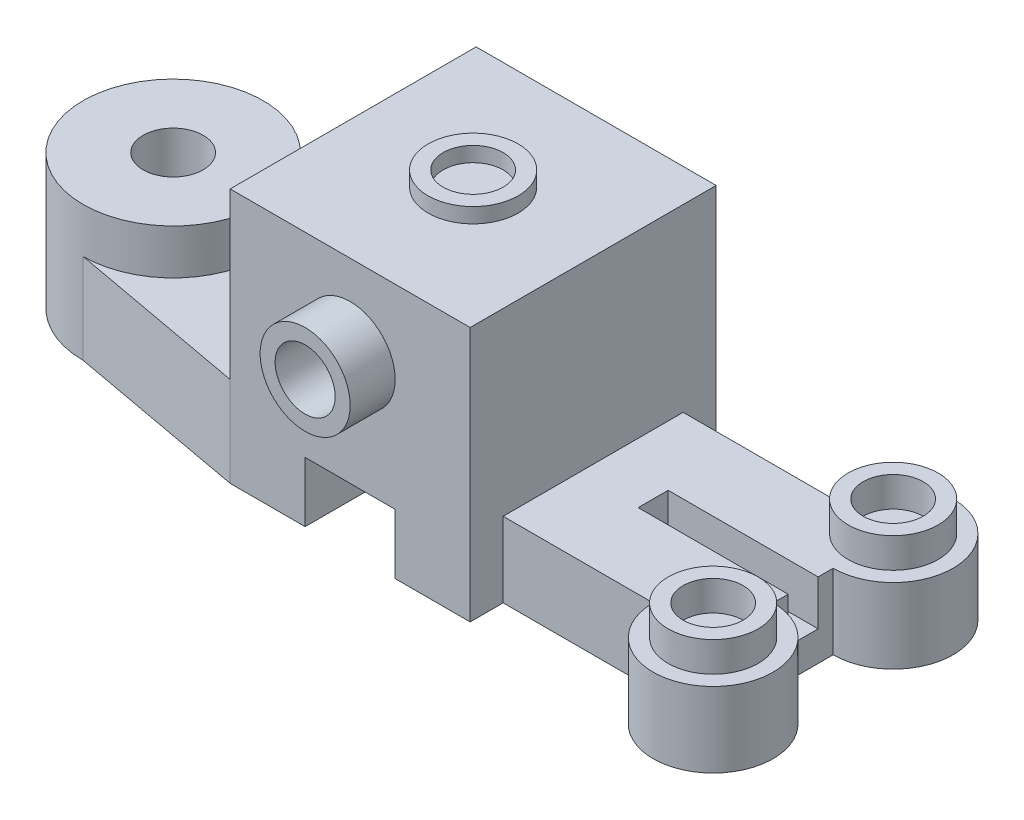
ISO-10303-21;
HEADER;
FILE_DESCRIPTION(('STEP AP214'),'2;1');
FILE_NAME('part.step','',(''),(''),'','','');
FILE_SCHEMA(('AUTOMOTIVE_DESIGN { 1 0 10303 214 1 1 1 1 }'));
ENDSEC;
DATA;
#1=APPLICATION_CONTEXT('core data for automotive mechanical design processes');
#2=APPLICATION_PROTOCOL_DEFINITION('international standard','automotive_design',2000,#1);
#3=PRODUCT_CONTEXT('',#1,'mechanical');
#4=PRODUCT('Part','Part','',(#3));
#5=PRODUCT_RELATED_PRODUCT_CATEGORY('part','',(#4));
#6=PRODUCT_DEFINITION_FORMATION('','',#4);
#7=PRODUCT_DEFINITION_CONTEXT('part definition',#1,'design');
#8=PRODUCT_DEFINITION('design','',#6,#7);
#9=PRODUCT_DEFINITION_SHAPE('','',#8);
#10=(LENGTH_UNIT() NAMED_UNIT(*) SI_UNIT(.MILLI.,.METRE.));
#11=(NAMED_UNIT(*) PLANE_ANGLE_UNIT() SI_UNIT($,.RADIAN.));
#12=(NAMED_UNIT(*) SI_UNIT($,.STERADIAN.) SOLID_ANGLE_UNIT());
#13=UNCERTAINTY_MEASURE_WITH_UNIT(LENGTH_MEASURE(1.E-05),#10,'distance_accuracy_value','');
#14=(GEOMETRIC_REPRESENTATION_CONTEXT(3) GLOBAL_UNCERTAINTY_ASSIGNED_CONTEXT((#13)) GLOBAL_UNIT_ASSIGNED_CONTEXT((#10,
#11,#12)) REPRESENTATION_CONTEXT('',''));
#15=CARTESIAN_POINT('',(0.,0.,0.));
#16=DIRECTION('',(0.,0.,1.));
#17=DIRECTION('',(1.,0.,0.));
#18=AXIS2_PLACEMENT_3D('',#15,#16,#17);
#19=CARTESIAN_POINT('',(80.,0.,82.));
#20=DIRECTION('',(-1.,0.,0.));
#21=DIRECTION('',(0.,0.,1.));
#22=AXIS2_PLACEMENT_3D('',#19,#20,#21);
#23=PLANE('',#22);
#24=DIRECTION('',(0.,-1.,0.));
#25=VECTOR('',#24,1.);
#26=CARTESIAN_POINT('',(80.,25.,71.));
#27=LINE('',#26,#25);
#28=CARTESIAN_POINT('',(80.,25.,71.));
#29=VERTEX_POINT('',#28);
#30=CARTESIAN_POINT('',(80.,0.,71.));
#31=VERTEX_POINT('',#30);
#32=EDGE_CURVE('E289',#29,#31,#27,.T.);
#33=ORIENTED_EDGE('',*,*,#32,.F.);
#34=DIRECTION('',(0.,0.,-1.));
#35=VECTOR('',#34,1.);
#36=CARTESIAN_POINT('',(80.,25.,71.));
#37=LINE('',#36,#35);
#38=CARTESIAN_POINT('',(80.,25.,11.));
#39=VERTEX_POINT('',#38);
#40=EDGE_CURVE('E271',#29,#39,#37,.T.);
#41=ORIENTED_EDGE('',*,*,#40,.T.);
#42=DIRECTION('',(0.,-1.,0.));
#43=VECTOR('',#42,1.);
#44=CARTESIAN_POINT('',(80.,25.,11.));
#45=LINE('',#44,#43);
#46=CARTESIAN_POINT('',(80.,0.,11.));
#47=VERTEX_POINT('',#46);
#48=EDGE_CURVE('E285',#39,#47,#45,.T.);
#49=ORIENTED_EDGE('',*,*,#48,.T.);
#50=DIRECTION('',(0.,0.,-1.));
#51=VECTOR('',#50,1.);
#52=CARTESIAN_POINT('',(80.,0.,82.));
#53=LINE('',#52,#51);
#54=CARTESIAN_POINT('',(80.,0.,0.));
#55=VERTEX_POINT('',#54);
#56=EDGE_CURVE('E375',#47,#55,#53,.T.);
#57=ORIENTED_EDGE('',*,*,#56,.T.);
#58=DIRECTION('',(0.,1.,0.));
#59=VECTOR('',#58,1.);
#60=CARTESIAN_POINT('',(80.,0.,0.));
#61=LINE('',#60,#59);
#62=CARTESIAN_POINT('',(80.,85.,0.));
#63=VERTEX_POINT('',#62);
#64=EDGE_CURVE('E364',#55,#63,#61,.T.);
#65=ORIENTED_EDGE('',*,*,#64,.T.);
#66=DIRECTION('',(0.,0.,-1.));
#67=VECTOR('',#66,1.);
#68=CARTESIAN_POINT('',(80.,85.,82.));
#69=LINE('',#68,#67);
#70=CARTESIAN_POINT('',(80.,85.,82.));
#71=VERTEX_POINT('',#70);
#72=EDGE_CURVE('E367',#71,#63,#69,.T.);
#73=ORIENTED_EDGE('',*,*,#72,.F.);
#74=DIRECTION('',(0.,1.,0.));
#75=VECTOR('',#74,1.);
#76=CARTESIAN_POINT('',(80.,0.,82.));
#77=LINE('',#76,#75);
#78=CARTESIAN_POINT('',(80.,0.,82.));
#79=VERTEX_POINT('',#78);
#80=EDGE_CURVE('E350',#79,#71,#77,.T.);
#81=ORIENTED_EDGE('',*,*,#80,.F.);
#82=EDGE_CURVE('E373',#79,#31,#53,.T.);
#83=ORIENTED_EDGE('',*,*,#82,.T.);
#84=EDGE_LOOP('',(#33,#41,#49,#57,#65,#73,#81,#83));
#85=FACE_BOUND('',#84,.T.);
#86=ADVANCED_FACE('F41',(#85),#23,.F.);
#87=CARTESIAN_POINT('',(0.,85.,82.));
#88=DIRECTION('',(1.,0.,0.));
#89=DIRECTION('',(0.,1.,0.));
#90=AXIS2_PLACEMENT_3D('',#87,#88,#89);
#91=PLANE('',#90);
#92=DIRECTION('',(0.,0.,-1.));
#93=VECTOR('',#92,1.);
#94=CARTESIAN_POINT('',(0.,30.,0.));
#95=LINE('',#94,#93);
#96=CARTESIAN_POINT('',(0.,30.,82.));
#97=VERTEX_POINT('',#96);
#98=CARTESIAN_POINT('',(0.,30.,0.));
#99=VERTEX_POINT('',#98);
#100=EDGE_CURVE('E304',#97,#99,#95,.T.);
#101=ORIENTED_EDGE('',*,*,#100,.F.);
#102=DIRECTION('',(0.,-1.,0.));
#103=VECTOR('',#102,1.);
#104=CARTESIAN_POINT('',(0.,85.,82.));
#105=LINE('',#104,#103);
#106=CARTESIAN_POINT('',(0.,85.,82.));
#107=VERTEX_POINT('',#106);
#108=EDGE_CURVE('E331',#107,#97,#105,.T.);
#109=ORIENTED_EDGE('',*,*,#108,.F.);
#110=DIRECTION('',(0.,0.,-1.));
#111=VECTOR('',#110,1.);
#112=CARTESIAN_POINT('',(0.,85.,82.));
#113=LINE('',#112,#111);
#114=CARTESIAN_POINT('',(0.,85.,0.));
#115=VERTEX_POINT('',#114);
#116=EDGE_CURVE('E353',#107,#115,#113,.T.);
#117=ORIENTED_EDGE('',*,*,#116,.T.);
#118=DIRECTION('',(0.,-1.,0.));
#119=VECTOR('',#118,1.);
#120=CARTESIAN_POINT('',(0.,85.,0.));
#121=LINE('',#120,#119);
#122=EDGE_CURVE('E335',#115,#99,#121,.T.);
#123=ORIENTED_EDGE('',*,*,#122,.T.);
#124=EDGE_LOOP('',(#101,#109,#117,#123));
#125=FACE_BOUND('',#124,.T.);
#126=ADVANCED_FACE('F43',(#125),#91,.F.);
#127=CARTESIAN_POINT('',(0.,0.,82.));
#128=DIRECTION('',(0.,1.,0.));
#129=DIRECTION('',(0.,0.,1.));
#130=AXIS2_PLACEMENT_3D('',#127,#128,#129);
#131=PLANE('',#130);
#132=DIRECTION('',(1.,0.,0.));
#133=VECTOR('',#132,1.);
#134=CARTESIAN_POINT('',(0.,0.,0.));
#135=LINE('',#134,#133);
#136=CARTESIAN_POINT('',(0.,0.,0.));
#137=VERTEX_POINT('',#136);
#138=CARTESIAN_POINT('',(25.,0.,0.));
#139=VERTEX_POINT('',#138);
#140=EDGE_CURVE('E351',#137,#139,#135,.T.);
#141=ORIENTED_EDGE('',*,*,#140,.T.);
#142=DIRECTION('',(0.,0.,-1.));
#143=VECTOR('',#142,1.);
#144=CARTESIAN_POINT('',(25.,0.,82.));
#145=LINE('',#144,#143);
#146=CARTESIAN_POINT('',(25.,0.,82.));
#147=VERTEX_POINT('',#146);
#148=EDGE_CURVE('E383',#147,#139,#145,.T.);
#149=ORIENTED_EDGE('',*,*,#148,.F.);
#150=DIRECTION('',(1.,0.,0.));
#151=VECTOR('',#150,1.);
#152=CARTESIAN_POINT('',(0.,0.,82.));
#153=LINE('',#152,#151);
#154=CARTESIAN_POINT('',(0.,0.,82.));
#155=VERTEX_POINT('',#154);
#156=EDGE_CURVE('E337',#155,#147,#153,.T.);
#157=ORIENTED_EDGE('',*,*,#156,.F.);
#158=DIRECTION('',(0.983606557377049,0.,0.180327868852459));
#159=VECTOR('',#158,1.);
#160=CARTESIAN_POINT('',(0.,0.,82.));
#161=LINE('',#160,#159);
#162=CARTESIAN_POINT('',(-60.,0.,71.));
#163=VERTEX_POINT('',#162);
#164=EDGE_CURVE('E307',#163,#155,#161,.T.);
#165=ORIENTED_EDGE('',*,*,#164,.F.);
#166=CARTESIAN_POINT('',(-60.,0.,41.));
#167=DIRECTION('',(0.,1.,0.));
#168=DIRECTION('',(0.,0.,1.));
#169=AXIS2_PLACEMENT_3D('',#166,#167,#168);
#170=CIRCLE('',#169,30.);
#171=CARTESIAN_POINT('',(-60.,0.,11.));
#172=VERTEX_POINT('',#171);
#173=EDGE_CURVE('E300',#172,#163,#170,.T.);
#174=ORIENTED_EDGE('',*,*,#173,.F.);
#175=DIRECTION('',(-0.983606557377049,0.,0.180327868852459));
#176=VECTOR('',#175,1.);
#177=CARTESIAN_POINT('',(0.,0.,0.));
#178=LINE('',#177,#176);
#179=EDGE_CURVE('E303',#137,#172,#178,.T.);
#180=ORIENTED_EDGE('',*,*,#179,.F.);
#181=EDGE_LOOP('',(#141,#149,#157,#165,#174,#180));
#182=FACE_BOUND('',#181,.T.);
#183=CARTESIAN_POINT('',(-60.,0.,41.));
#184=DIRECTION('',(0.,1.,0.));
#185=DIRECTION('',(0.,0.,1.));
#186=AXIS2_PLACEMENT_3D('',#183,#184,#185);
#187=CIRCLE('',#186,10.);
#188=CARTESIAN_POINT('',(-60.,0.,31.));
#189=VERTEX_POINT('',#188);
#190=EDGE_CURVE('E293',#189,#189,#187,.T.);
#191=ORIENTED_EDGE('',*,*,#190,.T.);
#192=EDGE_LOOP('',(#191));
#193=FACE_BOUND('',#192,.T.);
#194=ADVANCED_FACE('F451',(#182,#193),#131,.F.);
#195=CARTESIAN_POINT('',(25.,0.,82.));
#196=DIRECTION('',(-1.,0.,0.));
#197=DIRECTION('',(0.,0.,1.));
#198=AXIS2_PLACEMENT_3D('',#195,#196,#197);
#199=PLANE('',#198);
#200=DIRECTION('',(0.,1.,0.));
#201=VECTOR('',#200,1.);
#202=CARTESIAN_POINT('',(25.,0.,0.));
#203=LINE('',#202,#201);
#204=CARTESIAN_POINT('',(25.,20.,0.));
#205=VERTEX_POINT('',#204);
#206=EDGE_CURVE('E352',#139,#205,#203,.T.);
#207=ORIENTED_EDGE('',*,*,#206,.T.);
#208=DIRECTION('',(0.,0.,-1.));
#209=VECTOR('',#208,1.);
#210=CARTESIAN_POINT('',(25.,20.,82.));
#211=LINE('',#210,#209);
#212=CARTESIAN_POINT('',(25.,20.,82.));
#213=VERTEX_POINT('',#212);
#214=EDGE_CURVE('E385',#213,#205,#211,.T.);
#215=ORIENTED_EDGE('',*,*,#214,.F.);
#216=DIRECTION('',(0.,1.,0.));
#217=VECTOR('',#216,1.);
#218=CARTESIAN_POINT('',(25.,0.,82.));
#219=LINE('',#218,#217);
#220=EDGE_CURVE('E339',#147,#213,#219,.T.);
#221=ORIENTED_EDGE('',*,*,#220,.F.);
#222=ORIENTED_EDGE('',*,*,#148,.T.);
#223=EDGE_LOOP('',(#207,#215,#221,#222));
#224=FACE_BOUND('',#223,.T.);
#225=ADVANCED_FACE('F449',(#224),#199,.F.);
#226=CARTESIAN_POINT('',(25.,20.,82.));
#227=DIRECTION('',(0.,1.,0.));
#228=DIRECTION('',(0.,0.,1.));
#229=AXIS2_PLACEMENT_3D('',#226,#227,#228);
#230=PLANE('',#229);
#231=DIRECTION('',(1.,0.,0.));
#232=VECTOR('',#231,1.);
#233=CARTESIAN_POINT('',(25.,20.,0.));
#234=LINE('',#233,#232);
#235=CARTESIAN_POINT('',(55.,20.,0.));
#236=VERTEX_POINT('',#235);
#237=EDGE_CURVE('E357',#205,#236,#234,.T.);
#238=ORIENTED_EDGE('',*,*,#237,.T.);
#239=DIRECTION('',(0.,0.,-1.));
#240=VECTOR('',#239,1.);
#241=CARTESIAN_POINT('',(55.,20.,82.));
#242=LINE('',#241,#240);
#243=CARTESIAN_POINT('',(55.,20.,82.));
#244=VERTEX_POINT('',#243);
#245=EDGE_CURVE('E378',#244,#236,#242,.T.);
#246=ORIENTED_EDGE('',*,*,#245,.F.);
#247=DIRECTION('',(1.,0.,0.));
#248=VECTOR('',#247,1.);
#249=CARTESIAN_POINT('',(25.,20.,82.));
#250=LINE('',#249,#248);
#251=EDGE_CURVE('E344',#213,#244,#250,.T.);
#252=ORIENTED_EDGE('',*,*,#251,.F.);
#253=ORIENTED_EDGE('',*,*,#214,.T.);
#254=EDGE_LOOP('',(#238,#246,#252,#253));
#255=FACE_BOUND('',#254,.T.);
#256=ADVANCED_FACE('F444',(#255),#230,.F.);
#257=CARTESIAN_POINT('',(55.,20.,82.));
#258=DIRECTION('',(1.,0.,0.));
#259=DIRECTION('',(0.,0.,-1.));
#260=AXIS2_PLACEMENT_3D('',#257,#258,#259);
#261=PLANE('',#260);
#262=DIRECTION('',(0.,-1.,0.));
#263=VECTOR('',#262,1.);
#264=CARTESIAN_POINT('',(55.,20.,0.));
#265=LINE('',#264,#263);
#266=CARTESIAN_POINT('',(55.,0.,0.));
#267=VERTEX_POINT('',#266);
#268=EDGE_CURVE('E360',#236,#267,#265,.T.);
#269=ORIENTED_EDGE('',*,*,#268,.T.);
#270=DIRECTION('',(0.,0.,-1.));
#271=VECTOR('',#270,1.);
#272=CARTESIAN_POINT('',(55.,0.,82.));
#273=LINE('',#272,#271);
#274=CARTESIAN_POINT('',(55.,0.,82.));
#275=VERTEX_POINT('',#274);
#276=EDGE_CURVE('E376',#275,#267,#273,.T.);
#277=ORIENTED_EDGE('',*,*,#276,.F.);
#278=DIRECTION('',(0.,-1.,0.));
#279=VECTOR('',#278,1.);
#280=CARTESIAN_POINT('',(55.,20.,82.));
#281=LINE('',#280,#279);
#282=EDGE_CURVE('E345',#244,#275,#281,.T.);
#283=ORIENTED_EDGE('',*,*,#282,.F.);
#284=ORIENTED_EDGE('',*,*,#245,.T.);
#285=EDGE_LOOP('',(#269,#277,#283,#284));
#286=FACE_BOUND('',#285,.T.);
#287=ADVANCED_FACE('F441',(#286),#261,.F.);
#288=CARTESIAN_POINT('',(55.,0.,82.));
#289=DIRECTION('',(0.,1.,0.));
#290=DIRECTION('',(-1.,0.,0.));
#291=AXIS2_PLACEMENT_3D('',#288,#289,#290);
#292=PLANE('',#291);
#293=DIRECTION('',(0.,0.,1.));
#294=VECTOR('',#293,1.);
#295=CARTESIAN_POINT('',(150.,0.,11.));
#296=LINE('',#295,#294);
#297=CARTESIAN_POINT('',(150.,0.,31.));
#298=VERTEX_POINT('',#297);
#299=CARTESIAN_POINT('',(150.,0.,51.));
#300=VERTEX_POINT('',#299);
#301=EDGE_CURVE('E284',#298,#300,#296,.T.);
#302=ORIENTED_EDGE('',*,*,#301,.T.);
#303=CARTESIAN_POINT('',(150.,0.,71.));
#304=DIRECTION('',(0.,1.,0.));
#305=DIRECTION('',(0.,0.,1.));
#306=AXIS2_PLACEMENT_3D('',#303,#304,#305);
#307=CIRCLE('',#306,20.);
#308=CARTESIAN_POINT('',(130.,0.,71.));
#309=VERTEX_POINT('',#308);
#310=EDGE_CURVE('E249',#309,#300,#307,.T.);
#311=ORIENTED_EDGE('',*,*,#310,.F.);
#312=DIRECTION('',(-1.,0.,0.));
#313=VECTOR('',#312,1.);
#314=CARTESIAN_POINT('',(150.,0.,71.));
#315=LINE('',#314,#313);
#316=EDGE_CURVE('E63',#309,#31,#315,.T.);
#317=ORIENTED_EDGE('',*,*,#316,.T.);
#318=ORIENTED_EDGE('',*,*,#82,.F.);
#319=DIRECTION('',(1.,0.,0.));
#320=VECTOR('',#319,1.);
#321=CARTESIAN_POINT('',(55.,0.,82.));
#322=LINE('',#321,#320);
#323=EDGE_CURVE('E342',#275,#79,#322,.T.);
#324=ORIENTED_EDGE('',*,*,#323,.F.);
#325=ORIENTED_EDGE('',*,*,#276,.T.);
#326=DIRECTION('',(1.,0.,0.));
#327=VECTOR('',#326,1.);
#328=CARTESIAN_POINT('',(55.,0.,0.));
#329=LINE('',#328,#327);
#330=EDGE_CURVE('E363',#267,#55,#329,.T.);
#331=ORIENTED_EDGE('',*,*,#330,.T.);
#332=ORIENTED_EDGE('',*,*,#56,.F.);
#333=DIRECTION('',(1.,0.,0.));
#334=VECTOR('',#333,1.);
#335=CARTESIAN_POINT('',(80.,0.,11.));
#336=LINE('',#335,#334);
#337=CARTESIAN_POINT('',(130.,0.,11.));
#338=VERTEX_POINT('',#337);
#339=EDGE_CURVE('E275',#47,#338,#336,.T.);
#340=ORIENTED_EDGE('',*,*,#339,.T.);
#341=CARTESIAN_POINT('',(150.,0.,11.));
#342=DIRECTION('',(0.,1.,0.));
#343=DIRECTION('',(0.,0.,1.));
#344=AXIS2_PLACEMENT_3D('',#341,#342,#343);
#345=CIRCLE('',#344,20.);
#346=EDGE_CURVE('E261',#298,#338,#345,.T.);
#347=ORIENTED_EDGE('',*,*,#346,.F.);
#348=EDGE_LOOP('',(#302,#311,#317,#318,#324,#325,#331,#332,#340,#347));
#349=FACE_BOUND('',#348,.T.);
#350=ADVANCED_FACE('F405',(#349),#292,.F.);
#351=CARTESIAN_POINT('',(80.,85.,82.));
#352=DIRECTION('',(0.,-1.,0.));
#353=DIRECTION('',(1.,0.,0.));
#354=AXIS2_PLACEMENT_3D('',#351,#352,#353);
#355=PLANE('',#354);
#356=CARTESIAN_POINT('',(40.,85.,41.));
#357=DIRECTION('',(0.,-1.,0.));
#358=DIRECTION('',(1.,0.,0.));
#359=AXIS2_PLACEMENT_3D('',#356,#357,#358);
#360=CIRCLE('',#359,15.);
#361=CARTESIAN_POINT('',(55.,85.,41.));
#362=VERTEX_POINT('',#361);
#363=EDGE_CURVE('E47',#362,#362,#360,.F.);
#364=ORIENTED_EDGE('',*,*,#363,.F.);
#365=EDGE_LOOP('',(#364));
#366=FACE_BOUND('',#365,.T.);
#367=DIRECTION('',(-1.,0.,0.));
#368=VECTOR('',#367,1.);
#369=CARTESIAN_POINT('',(80.,85.,0.));
#370=LINE('',#369,#368);
#371=EDGE_CURVE('E340',#63,#115,#370,.T.);
#372=ORIENTED_EDGE('',*,*,#371,.T.);
#373=ORIENTED_EDGE('',*,*,#116,.F.);
#374=DIRECTION('',(-1.,0.,0.));
#375=VECTOR('',#374,1.);
#376=CARTESIAN_POINT('',(80.,85.,82.));
#377=LINE('',#376,#375);
#378=EDGE_CURVE('E347',#71,#107,#377,.T.);
#379=ORIENTED_EDGE('',*,*,#378,.F.);
#380=ORIENTED_EDGE('',*,*,#72,.T.);
#381=EDGE_LOOP('',(#372,#373,#379,#380));
#382=FACE_BOUND('',#381,.T.);
#383=ADVANCED_FACE('F396',(#366,#382),#355,.F.);
#384=CARTESIAN_POINT('',(0.,0.,82.));
#385=DIRECTION('',(0.,0.,1.));
#386=DIRECTION('',(1.,0.,0.));
#387=AXIS2_PLACEMENT_3D('',#384,#385,#386);
#388=PLANE('',#387);
#389=CARTESIAN_POINT('',(40.,57.5,82.));
#390=DIRECTION('',(0.,0.,1.));
#391=DIRECTION('',(1.,0.,0.));
#392=AXIS2_PLACEMENT_3D('',#389,#390,#391);
#393=CIRCLE('',#392,15.);
#394=CARTESIAN_POINT('',(55.,57.5,82.));
#395=VERTEX_POINT('',#394);
#396=EDGE_CURVE('E212',#395,#395,#393,.T.);
#397=ORIENTED_EDGE('',*,*,#396,.F.);
#398=EDGE_LOOP('',(#397));
#399=FACE_BOUND('',#398,.T.);
#400=ORIENTED_EDGE('',*,*,#108,.T.);
#401=DIRECTION('',(0.,-1.,0.));
#402=VECTOR('',#401,1.);
#403=CARTESIAN_POINT('',(0.,30.,82.));
#404=LINE('',#403,#402);
#405=EDGE_CURVE('E319',#97,#155,#404,.T.);
#406=ORIENTED_EDGE('',*,*,#405,.T.);
#407=ORIENTED_EDGE('',*,*,#156,.T.);
#408=ORIENTED_EDGE('',*,*,#220,.T.);
#409=ORIENTED_EDGE('',*,*,#251,.T.);
#410=ORIENTED_EDGE('',*,*,#282,.T.);
#411=ORIENTED_EDGE('',*,*,#323,.T.);
#412=ORIENTED_EDGE('',*,*,#80,.T.);
#413=ORIENTED_EDGE('',*,*,#378,.T.);
#414=EDGE_LOOP('',(#400,#406,#407,#408,#409,#410,#411,#412,#413));
#415=FACE_BOUND('',#414,.T.);
#416=ADVANCED_FACE('F402',(#399,#415),#388,.T.);
#417=CARTESIAN_POINT('',(0.,0.,0.));
#418=DIRECTION('',(0.,0.,1.));
#419=DIRECTION('',(1.,0.,0.));
#420=AXIS2_PLACEMENT_3D('',#417,#418,#419);
#421=PLANE('',#420);
#422=ORIENTED_EDGE('',*,*,#122,.F.);
#423=ORIENTED_EDGE('',*,*,#371,.F.);
#424=ORIENTED_EDGE('',*,*,#64,.F.);
#425=ORIENTED_EDGE('',*,*,#330,.F.);
#426=ORIENTED_EDGE('',*,*,#268,.F.);
#427=ORIENTED_EDGE('',*,*,#237,.F.);
#428=ORIENTED_EDGE('',*,*,#206,.F.);
#429=ORIENTED_EDGE('',*,*,#140,.F.);
#430=DIRECTION('',(0.,-1.,0.));
#431=VECTOR('',#430,1.);
#432=CARTESIAN_POINT('',(0.,30.,0.));
#433=LINE('',#432,#431);
#434=EDGE_CURVE('E327',#99,#137,#433,.T.);
#435=ORIENTED_EDGE('',*,*,#434,.F.);
#436=EDGE_LOOP('',(#422,#423,#424,#425,#426,#427,#428,#429,#435));
#437=FACE_BOUND('',#436,.T.);
#438=ADVANCED_FACE('F414',(#437),#421,.F.);
#439=CARTESIAN_POINT('',(0.,30.,0.));
#440=DIRECTION('',(0.180327868852459,0.,0.983606557377049));
#441=DIRECTION('',(0.983606557377049,0.,-0.180327868852459));
#442=AXIS2_PLACEMENT_3D('',#439,#440,#441);
#443=PLANE('',#442);
#444=ORIENTED_EDGE('',*,*,#179,.T.);
#445=DIRECTION('',(0.,-1.,0.));
#446=VECTOR('',#445,1.);
#447=CARTESIAN_POINT('',(-60.,30.,11.));
#448=LINE('',#447,#446);
#449=CARTESIAN_POINT('',(-60.0000000000001,30.,11.));
#450=VERTEX_POINT('',#449);
#451=EDGE_CURVE('E330',#450,#172,#448,.T.);
#452=ORIENTED_EDGE('',*,*,#451,.F.);
#453=DIRECTION('',(-0.983606557377049,0.,0.180327868852459));
#454=VECTOR('',#453,1.);
#455=CARTESIAN_POINT('',(0.,30.,0.));
#456=LINE('',#455,#454);
#457=EDGE_CURVE('E308',#99,#450,#456,.T.);
#458=ORIENTED_EDGE('',*,*,#457,.F.);
#459=ORIENTED_EDGE('',*,*,#434,.T.);
#460=EDGE_LOOP('',(#444,#452,#458,#459));
#461=FACE_BOUND('',#460,.T.);
#462=ADVANCED_FACE('F423',(#461),#443,.F.);
#463=CARTESIAN_POINT('',(0.,30.,82.));
#464=DIRECTION('',(0.180327868852459,0.,-0.983606557377049));
#465=DIRECTION('',(-0.983606557377049,0.,-0.180327868852459));
#466=AXIS2_PLACEMENT_3D('',#463,#464,#465);
#467=PLANE('',#466);
#468=ORIENTED_EDGE('',*,*,#164,.T.);
#469=ORIENTED_EDGE('',*,*,#405,.F.);
#470=DIRECTION('',(0.983606557377049,0.,0.180327868852459));
#471=VECTOR('',#470,1.);
#472=CARTESIAN_POINT('',(0.,30.,82.));
#473=LINE('',#472,#471);
#474=CARTESIAN_POINT('',(-60.,30.,71.));
#475=VERTEX_POINT('',#474);
#476=EDGE_CURVE('E314',#475,#97,#473,.T.);
#477=ORIENTED_EDGE('',*,*,#476,.F.);
#478=DIRECTION('',(0.,-1.,0.));
#479=VECTOR('',#478,1.);
#480=CARTESIAN_POINT('',(-60.,30.,71.));
#481=LINE('',#480,#479);
#482=EDGE_CURVE('E323',#475,#163,#481,.T.);
#483=ORIENTED_EDGE('',*,*,#482,.T.);
#484=EDGE_LOOP('',(#468,#469,#477,#483));
#485=FACE_BOUND('',#484,.T.);
#486=ADVANCED_FACE('F457',(#485),#467,.F.);
#487=CARTESIAN_POINT('',(-60.0000000000001,30.,41.));
#488=DIRECTION('',(0.,-1.,0.));
#489=DIRECTION('',(0.,0.,-1.));
#490=AXIS2_PLACEMENT_3D('',#487,#488,#489);
#491=PLANE('',#490);
#492=ORIENTED_EDGE('',*,*,#100,.T.);
#493=ORIENTED_EDGE('',*,*,#457,.T.);
#494=CARTESIAN_POINT('',(-60.0000000000001,30.,41.));
#495=DIRECTION('',(0.,-1.,0.));
#496=DIRECTION('',(0.,0.,-1.));
#497=AXIS2_PLACEMENT_3D('',#494,#495,#496);
#498=CIRCLE('',#497,30.);
#499=EDGE_CURVE('E315',#450,#475,#498,.T.);
#500=ORIENTED_EDGE('',*,*,#499,.T.);
#501=ORIENTED_EDGE('',*,*,#476,.T.);
#502=EDGE_LOOP('',(#492,#493,#500,#501));
#503=FACE_BOUND('',#502,.T.);
#504=ADVANCED_FACE('F421',(#503),#491,.F.);
#505=CARTESIAN_POINT('',(-60.,45.,41.));
#506=DIRECTION('',(0.,-1.,0.));
#507=DIRECTION('',(0.,0.,-1.));
#508=AXIS2_PLACEMENT_3D('',#505,#506,#507);
#509=CYLINDRICAL_SURFACE('',#508,30.);
#510=CARTESIAN_POINT('',(-60.,45.,41.));
#511=DIRECTION('',(0.,1.,0.));
#512=DIRECTION('',(0.,0.,1.));
#513=AXIS2_PLACEMENT_3D('',#510,#511,#512);
#514=CIRCLE('',#513,30.);
#515=CARTESIAN_POINT('',(-60.,45.,71.));
#516=VERTEX_POINT('',#515);
#517=EDGE_CURVE('E297',#516,#516,#514,.T.);
#518=ORIENTED_EDGE('',*,*,#517,.F.);
#519=EDGE_LOOP('',(#518));
#520=FACE_BOUND('',#519,.T.);
#521=ORIENTED_EDGE('',*,*,#499,.F.);
#522=ORIENTED_EDGE('',*,*,#451,.T.);
#523=ORIENTED_EDGE('',*,*,#173,.T.);
#524=ORIENTED_EDGE('',*,*,#482,.F.);
#525=EDGE_LOOP('',(#521,#522,#523,#524));
#526=FACE_BOUND('',#525,.T.);
#527=ADVANCED_FACE('F460',(#520,#526),#509,.T.);
#528=CARTESIAN_POINT('',(-60.,45.,41.));
#529=DIRECTION('',(0.,1.,0.));
#530=DIRECTION('',(0.,0.,1.));
#531=AXIS2_PLACEMENT_3D('',#528,#529,#530);
#532=PLANE('',#531);
#533=ORIENTED_EDGE('',*,*,#517,.T.);
#534=EDGE_LOOP('',(#533));
#535=FACE_BOUND('',#534,.T.);
#536=CARTESIAN_POINT('',(-60.,45.,41.));
#537=DIRECTION('',(0.,1.,0.));
#538=DIRECTION('',(0.,0.,1.));
#539=AXIS2_PLACEMENT_3D('',#536,#537,#538);
#540=CIRCLE('',#539,10.);
#541=CARTESIAN_POINT('',(-60.,45.,31.));
#542=VERTEX_POINT('',#541);
#543=EDGE_CURVE('E295',#542,#542,#540,.T.);
#544=ORIENTED_EDGE('',*,*,#543,.F.);
#545=EDGE_LOOP('',(#544));
#546=FACE_BOUND('',#545,.T.);
#547=ADVANCED_FACE('F803',(#535,#546),#532,.T.);
#548=CARTESIAN_POINT('',(-60.,45.,41.));
#549=DIRECTION('',(0.,-1.,0.));
#550=DIRECTION('',(0.,0.,-1.));
#551=AXIS2_PLACEMENT_3D('',#548,#549,#550);
#552=CYLINDRICAL_SURFACE('',#551,10.);
#553=CARTESIAN_POINT('',(-60.,45.,31.));
#554=CARTESIAN_POINT('',(-60.,44.53125,31.));
#555=CARTESIAN_POINT('',(-60.,44.0625,31.));
#556=CARTESIAN_POINT('',(-60.,43.125,31.));
#557=CARTESIAN_POINT('',(-60.,42.65625,31.));
#558=CARTESIAN_POINT('',(-60.,41.71875,31.));
#559=CARTESIAN_POINT('',(-60.,41.25,31.));
#560=CARTESIAN_POINT('',(-60.,40.3125,31.));
#561=CARTESIAN_POINT('',(-60.,39.84375,31.));
#562=CARTESIAN_POINT('',(-60.,38.90625,31.));
#563=CARTESIAN_POINT('',(-60.,38.4375,31.));
#564=CARTESIAN_POINT('',(-60.,37.5,31.));
#565=CARTESIAN_POINT('',(-60.,37.03125,31.));
#566=CARTESIAN_POINT('',(-60.,36.09375,31.));
#567=CARTESIAN_POINT('',(-60.,35.625,31.));
#568=CARTESIAN_POINT('',(-60.,34.6875,31.));
#569=CARTESIAN_POINT('',(-60.,34.21875,31.));
#570=CARTESIAN_POINT('',(-60.,33.28125,31.));
#571=CARTESIAN_POINT('',(-60.,32.8125,31.));
#572=CARTESIAN_POINT('',(-60.,31.875,31.));
#573=CARTESIAN_POINT('',(-60.,31.40625,31.));
#574=CARTESIAN_POINT('',(-60.,30.46875,31.));
#575=CARTESIAN_POINT('',(-60.,30.,31.));
#576=CARTESIAN_POINT('',(-60.,29.0625,31.));
#577=CARTESIAN_POINT('',(-60.,28.59375,31.));
#578=CARTESIAN_POINT('',(-60.,27.65625,31.));
#579=CARTESIAN_POINT('',(-60.,27.1875,31.));
#580=CARTESIAN_POINT('',(-60.,26.25,31.));
#581=CARTESIAN_POINT('',(-60.,25.78125,31.));
#582=CARTESIAN_POINT('',(-60.,24.84375,31.));
#583=CARTESIAN_POINT('',(-60.,24.375,31.));
#584=CARTESIAN_POINT('',(-60.,23.4375,31.));
#585=CARTESIAN_POINT('',(-60.,22.96875,31.));
#586=CARTESIAN_POINT('',(-60.,22.03125,31.));
#587=CARTESIAN_POINT('',(-60.,21.5625,31.));
#588=CARTESIAN_POINT('',(-60.,20.625,31.));
#589=CARTESIAN_POINT('',(-60.,20.15625,31.));
#590=CARTESIAN_POINT('',(-60.,19.21875,31.));
#591=CARTESIAN_POINT('',(-60.,18.75,31.));
#592=CARTESIAN_POINT('',(-60.,17.8125,31.));
#593=CARTESIAN_POINT('',(-60.,17.34375,31.));
#594=CARTESIAN_POINT('',(-60.,16.40625,31.));
#595=CARTESIAN_POINT('',(-60.,15.9375,31.));
#596=CARTESIAN_POINT('',(-60.,15.,31.));
#597=CARTESIAN_POINT('',(-60.,14.53125,31.));
#598=CARTESIAN_POINT('',(-60.,13.59375,31.));
#599=CARTESIAN_POINT('',(-60.,13.125,31.));
#600=CARTESIAN_POINT('',(-60.,12.1875,31.));
#601=CARTESIAN_POINT('',(-60.,11.71875,31.));
#602=CARTESIAN_POINT('',(-60.,10.78125,31.));
#603=CARTESIAN_POINT('',(-60.,10.3125,31.));
#604=CARTESIAN_POINT('',(-60.,9.375,31.));
#605=CARTESIAN_POINT('',(-60.,8.90625,31.));
#606=CARTESIAN_POINT('',(-60.,7.96874999999999,31.));
#607=CARTESIAN_POINT('',(-60.,7.5,31.));
#608=CARTESIAN_POINT('',(-60.,6.5625,31.));
#609=CARTESIAN_POINT('',(-60.,6.09375,31.));
#610=CARTESIAN_POINT('',(-60.,5.15625,31.));
#611=CARTESIAN_POINT('',(-60.,4.68749999999999,31.));
#612=CARTESIAN_POINT('',(-60.,3.74999999999999,31.));
#613=CARTESIAN_POINT('',(-60.,3.28124999999999,31.));
#614=CARTESIAN_POINT('',(-60.,2.34374999999999,31.));
#615=CARTESIAN_POINT('',(-60.,1.87499999999999,31.));
#616=CARTESIAN_POINT('',(-60.,0.937499999999992,31.));
#617=CARTESIAN_POINT('',(-60.,0.468749999999993,31.));
#618=CARTESIAN_POINT('',(-60.,0.,31.));
#619=B_SPLINE_CURVE_WITH_KNOTS('',3,(#553,#554,#555,#556,#557,#558,#559,#560,#561,#562,#563,
#564,#565,#566,#567,#568,#569,#570,#571,#572,#573,#574,#575,#576,#577,#578,#579,#580,#581,#582,
#583,#584,#585,#586,#587,#588,#589,#590,#591,#592,#593,#594,#595,#596,#597,#598,#599,#600,#601,
#602,#603,#604,#605,#606,#607,#608,#609,#610,#611,#612,#613,#614,#615,#616,#617,#618),
.UNSPECIFIED.,.F.,.F.,(4,2,2,2,2,2,2,2,2,2,2,2,2,2,2,2,2,2,2,2,2,2,2,2,2,2,2,2,2,2,2,2,4),(0.,
1.40625,2.8125,4.21875000000001,5.62500000000001,7.03125,8.4375,9.84375000000001,11.25,12.65625,
14.0625,15.46875,16.875,18.28125,19.6875,21.09375,22.5,23.90625,25.3125,26.71875,28.125,
29.53125,30.9375,32.34375,33.75,35.15625,36.5625,37.96875,39.375,40.78125,42.1875,43.59375,45.),.UNSPECIFIED.);
#620=EDGE_CURVE('BSEAM545',#542,#189,#619,.T.);
#621=ORIENTED_EDGE('',*,*,#543,.T.);
#622=ORIENTED_EDGE('',*,*,#190,.F.);
#623=ORIENTED_EDGE('',*,*,#620,.T.);
#624=ORIENTED_EDGE('',*,*,#620,.F.);
#625=EDGE_LOOP('',(#621,#623,#622,#624));
#626=FACE_BOUND('',#625,.T.);
#627=ADVANCED_FACE('F545',(#626),#552,.F.);
#628=CARTESIAN_POINT('',(150.,25.,71.));
#629=DIRECTION('',(0.,0.,1.));
#630=DIRECTION('',(1.,0.,0.));
#631=AXIS2_PLACEMENT_3D('',#628,#629,#630);
#632=PLANE('',#631);
#633=DIRECTION('',(0.,1.,0.));
#634=VECTOR('',#633,1.);
#635=CARTESIAN_POINT('',(130.,0.,71.));
#636=LINE('',#635,#634);
#637=CARTESIAN_POINT('',(130.,25.,71.));
#638=VERTEX_POINT('',#637);
#639=EDGE_CURVE('E260',#638,#309,#636,.F.);
#640=ORIENTED_EDGE('',*,*,#639,.F.);
#641=DIRECTION('',(-1.,0.,0.));
#642=VECTOR('',#641,1.);
#643=CARTESIAN_POINT('',(150.,25.,71.));
#644=LINE('',#643,#642);
#645=EDGE_CURVE('E277',#638,#29,#644,.T.);
#646=ORIENTED_EDGE('',*,*,#645,.T.);
#647=ORIENTED_EDGE('',*,*,#32,.T.);
#648=ORIENTED_EDGE('',*,*,#316,.F.);
#649=EDGE_LOOP('',(#640,#646,#647,#648));
#650=FACE_BOUND('',#649,.T.);
#651=ADVANCED_FACE('F536',(#650),#632,.T.);
#652=CARTESIAN_POINT('',(150.,25.,11.));
#653=DIRECTION('',(1.,0.,0.));
#654=DIRECTION('',(0.,0.,-1.));
#655=AXIS2_PLACEMENT_3D('',#652,#653,#654);
#656=PLANE('',#655);
#657=DIRECTION('',(0.,1.,0.));
#658=VECTOR('',#657,1.);
#659=CARTESIAN_POINT('',(150.,10.,46.));
#660=LINE('',#659,#658);
#661=CARTESIAN_POINT('',(150.,10.,46.));
#662=VERTEX_POINT('',#661);
#663=CARTESIAN_POINT('',(150.,25.,46.));
#664=VERTEX_POINT('',#663);
#665=EDGE_CURVE('E216',#662,#664,#660,.T.);
#666=ORIENTED_EDGE('',*,*,#665,.T.);
#667=DIRECTION('',(0.,0.,1.));
#668=VECTOR('',#667,1.);
#669=CARTESIAN_POINT('',(150.,25.,11.));
#670=LINE('',#669,#668);
#671=CARTESIAN_POINT('',(150.,25.,51.));
#672=VERTEX_POINT('',#671);
#673=EDGE_CURVE('E280',#664,#672,#670,.T.);
#674=ORIENTED_EDGE('',*,*,#673,.T.);
#675=DIRECTION('',(0.,1.,0.));
#676=VECTOR('',#675,1.);
#677=CARTESIAN_POINT('',(150.,0.,51.));
#678=LINE('',#677,#676);
#679=EDGE_CURVE('E254',#300,#672,#678,.T.);
#680=ORIENTED_EDGE('',*,*,#679,.F.);
#681=ORIENTED_EDGE('',*,*,#301,.F.);
#682=DIRECTION('',(0.,1.,0.));
#683=VECTOR('',#682,1.);
#684=CARTESIAN_POINT('',(150.,0.,31.));
#685=LINE('',#684,#683);
#686=CARTESIAN_POINT('',(150.,25.,31.));
#687=VERTEX_POINT('',#686);
#688=EDGE_CURVE('E269',#687,#298,#685,.F.);
#689=ORIENTED_EDGE('',*,*,#688,.F.);
#690=CARTESIAN_POINT('',(150.,25.,36.));
#691=VERTEX_POINT('',#690);
#692=EDGE_CURVE('E202',#687,#691,#670,.T.);
#693=ORIENTED_EDGE('',*,*,#692,.T.);
#694=DIRECTION('',(0.,1.,0.));
#695=VECTOR('',#694,1.);
#696=CARTESIAN_POINT('',(150.,10.,36.));
#697=LINE('',#696,#695);
#698=CARTESIAN_POINT('',(150.,10.,36.));
#699=VERTEX_POINT('',#698);
#700=EDGE_CURVE('E57',#699,#691,#697,.T.);
#701=ORIENTED_EDGE('',*,*,#700,.F.);
#702=DIRECTION('',(0.,0.,-1.));
#703=VECTOR('',#702,1.);
#704=CARTESIAN_POINT('',(150.,10.,46.));
#705=LINE('',#704,#703);
#706=EDGE_CURVE('E190',#662,#699,#705,.T.);
#707=ORIENTED_EDGE('',*,*,#706,.F.);
#708=EDGE_LOOP('',(#666,#674,#680,#681,#689,#693,#701,#707));
#709=FACE_BOUND('',#708,.T.);
#710=ADVANCED_FACE('F201',(#709),#656,.T.);
#711=CARTESIAN_POINT('',(80.,25.,11.));
#712=DIRECTION('',(0.,0.,-1.));
#713=DIRECTION('',(-1.,0.,0.));
#714=AXIS2_PLACEMENT_3D('',#711,#712,#713);
#715=PLANE('',#714);
#716=DIRECTION('',(0.,1.,0.));
#717=VECTOR('',#716,1.);
#718=CARTESIAN_POINT('',(130.,0.,11.));
#719=LINE('',#718,#717);
#720=CARTESIAN_POINT('',(130.,25.,11.));
#721=VERTEX_POINT('',#720);
#722=EDGE_CURVE('E262',#338,#721,#719,.T.);
#723=ORIENTED_EDGE('',*,*,#722,.F.);
#724=ORIENTED_EDGE('',*,*,#339,.F.);
#725=ORIENTED_EDGE('',*,*,#48,.F.);
#726=DIRECTION('',(1.,0.,0.));
#727=VECTOR('',#726,1.);
#728=CARTESIAN_POINT('',(80.,25.,11.));
#729=LINE('',#728,#727);
#730=EDGE_CURVE('E279',#39,#721,#729,.T.);
#731=ORIENTED_EDGE('',*,*,#730,.T.);
#732=EDGE_LOOP('',(#723,#724,#725,#731));
#733=FACE_BOUND('',#732,.T.);
#734=ADVANCED_FACE('F552',(#733),#715,.T.);
#735=CARTESIAN_POINT('',(0.,25.,0.));
#736=DIRECTION('',(0.,-1.,0.));
#737=DIRECTION('',(0.,0.,-1.));
#738=AXIS2_PLACEMENT_3D('',#735,#736,#737);
#739=PLANE('',#738);
#740=CARTESIAN_POINT('',(150.,25.,71.));
#741=DIRECTION('',(0.,-1.,0.));
#742=DIRECTION('',(0.,0.,-1.));
#743=AXIS2_PLACEMENT_3D('',#740,#741,#742);
#744=CIRCLE('',#743,15.);
#745=CARTESIAN_POINT('',(150.,25.,56.));
#746=VERTEX_POINT('',#745);
#747=EDGE_CURVE('E391',#746,#746,#744,.F.);
#748=ORIENTED_EDGE('',*,*,#747,.F.);
#749=EDGE_LOOP('',(#748));
#750=FACE_BOUND('',#749,.T.);
#751=CARTESIAN_POINT('',(150.,25.,11.));
#752=DIRECTION('',(0.,-1.,0.));
#753=DIRECTION('',(0.,0.,-1.));
#754=AXIS2_PLACEMENT_3D('',#751,#752,#753);
#755=CIRCLE('',#754,15.);
#756=CARTESIAN_POINT('',(150.,25.,-4.));
#757=VERTEX_POINT('',#756);
#758=EDGE_CURVE('E390',#757,#757,#755,.F.);
#759=ORIENTED_EDGE('',*,*,#758,.F.);
#760=EDGE_LOOP('',(#759));
#761=FACE_BOUND('',#760,.T.);
#762=ORIENTED_EDGE('',*,*,#673,.F.);
#763=DIRECTION('',(1.,0.,0.));
#764=VECTOR('',#763,1.);
#765=CARTESIAN_POINT('',(100.,25.,46.));
#766=LINE('',#765,#764);
#767=CARTESIAN_POINT('',(100.,25.,46.));
#768=VERTEX_POINT('',#767);
#769=EDGE_CURVE('E192',#768,#664,#766,.T.);
#770=ORIENTED_EDGE('',*,*,#769,.F.);
#771=DIRECTION('',(0.,0.,1.));
#772=VECTOR('',#771,1.);
#773=CARTESIAN_POINT('',(100.,25.,36.));
#774=LINE('',#773,#772);
#775=CARTESIAN_POINT('',(100.,25.,36.));
#776=VERTEX_POINT('',#775);
#777=EDGE_CURVE('E877',#776,#768,#774,.T.);
#778=ORIENTED_EDGE('',*,*,#777,.F.);
#779=DIRECTION('',(-1.,0.,0.));
#780=VECTOR('',#779,1.);
#781=CARTESIAN_POINT('',(150.,25.,36.));
#782=LINE('',#781,#780);
#783=EDGE_CURVE('E879',#691,#776,#782,.T.);
#784=ORIENTED_EDGE('',*,*,#783,.F.);
#785=ORIENTED_EDGE('',*,*,#692,.F.);
#786=CARTESIAN_POINT('',(150.,25.,11.));
#787=DIRECTION('',(0.,1.,0.));
#788=DIRECTION('',(0.,0.,1.));
#789=AXIS2_PLACEMENT_3D('',#786,#787,#788);
#790=CIRCLE('',#789,20.);
#791=EDGE_CURVE('E257',#687,#721,#790,.T.);
#792=ORIENTED_EDGE('',*,*,#791,.T.);
#793=ORIENTED_EDGE('',*,*,#730,.F.);
#794=ORIENTED_EDGE('',*,*,#40,.F.);
#795=ORIENTED_EDGE('',*,*,#645,.F.);
#796=CARTESIAN_POINT('',(150.,25.,71.));
#797=DIRECTION('',(0.,1.,0.));
#798=DIRECTION('',(0.,0.,1.));
#799=AXIS2_PLACEMENT_3D('',#796,#797,#798);
#800=CIRCLE('',#799,20.);
#801=EDGE_CURVE('E248',#638,#672,#800,.T.);
#802=ORIENTED_EDGE('',*,*,#801,.T.);
#803=EDGE_LOOP('',(#762,#770,#778,#784,#785,#792,#793,#794,#795,#802));
#804=FACE_BOUND('',#803,.T.);
#805=ADVANCED_FACE('F561',(#750,#761,#804),#739,.F.);
#806=CARTESIAN_POINT('',(150.,0.,11.));
#807=DIRECTION('',(0.,1.,0.));
#808=DIRECTION('',(0.,0.,1.));
#809=AXIS2_PLACEMENT_3D('',#806,#807,#808);
#810=CYLINDRICAL_SURFACE('',#809,20.);
#811=ORIENTED_EDGE('',*,*,#791,.F.);
#812=ORIENTED_EDGE('',*,*,#688,.T.);
#813=ORIENTED_EDGE('',*,*,#346,.T.);
#814=ORIENTED_EDGE('',*,*,#722,.T.);
#815=EDGE_LOOP('',(#811,#812,#813,#814));
#816=FACE_BOUND('',#815,.T.);
#817=ADVANCED_FACE('F571',(#816),#810,.T.);
#818=CARTESIAN_POINT('',(150.,0.,71.));
#819=DIRECTION('',(0.,1.,0.));
#820=DIRECTION('',(0.,0.,1.));
#821=AXIS2_PLACEMENT_3D('',#818,#819,#820);
#822=CYLINDRICAL_SURFACE('',#821,20.);
#823=ORIENTED_EDGE('',*,*,#801,.F.);
#824=ORIENTED_EDGE('',*,*,#639,.T.);
#825=ORIENTED_EDGE('',*,*,#310,.T.);
#826=ORIENTED_EDGE('',*,*,#679,.T.);
#827=EDGE_LOOP('',(#823,#824,#825,#826));
#828=FACE_BOUND('',#827,.T.);
#829=ADVANCED_FACE('F595',(#828),#822,.T.);
#830=CARTESIAN_POINT('',(150.,35.,11.));
#831=DIRECTION('',(0.,1.,0.));
#832=DIRECTION('',(0.,0.,1.));
#833=AXIS2_PLACEMENT_3D('',#830,#831,#832);
#834=PLANE('',#833);
#835=CARTESIAN_POINT('',(150.,35.,11.));
#836=DIRECTION('',(0.,1.,0.));
#837=DIRECTION('',(0.,0.,1.));
#838=AXIS2_PLACEMENT_3D('',#835,#836,#837);
#839=CIRCLE('',#838,15.);
#840=CARTESIAN_POINT('',(150.,35.,26.));
#841=VERTEX_POINT('',#840);
#842=EDGE_CURVE('E242',#841,#841,#839,.T.);
#843=ORIENTED_EDGE('',*,*,#842,.T.);
#844=EDGE_LOOP('',(#843));
#845=FACE_BOUND('',#844,.T.);
#846=CARTESIAN_POINT('',(150.,35.,11.));
#847=DIRECTION('',(0.,1.,0.));
#848=DIRECTION('',(0.,0.,1.));
#849=AXIS2_PLACEMENT_3D('',#846,#847,#848);
#850=CIRCLE('',#849,10.);
#851=CARTESIAN_POINT('',(150.,35.,21.));
#852=VERTEX_POINT('',#851);
#853=EDGE_CURVE('E241',#852,#852,#850,.T.);
#854=ORIENTED_EDGE('',*,*,#853,.F.);
#855=EDGE_LOOP('',(#854));
#856=FACE_BOUND('',#855,.T.);
#857=ADVANCED_FACE('F601',(#845,#856),#834,.T.);
#858=CARTESIAN_POINT('',(150.,35.,11.));
#859=DIRECTION('',(0.,-1.,0.));
#860=DIRECTION('',(0.,0.,-1.));
#861=AXIS2_PLACEMENT_3D('',#858,#859,#860);
#862=CYLINDRICAL_SURFACE('',#861,15.);
#863=ORIENTED_EDGE('',*,*,#842,.F.);
#864=EDGE_LOOP('',(#863));
#865=FACE_BOUND('',#864,.T.);
#866=ORIENTED_EDGE('',*,*,#758,.T.);
#867=EDGE_LOOP('',(#866));
#868=FACE_BOUND('',#867,.T.);
#869=ADVANCED_FACE('F645',(#865,#868),#862,.T.);
#870=CARTESIAN_POINT('',(150.,35.,11.));
#871=DIRECTION('',(0.,-1.,0.));
#872=DIRECTION('',(0.,0.,-1.));
#873=AXIS2_PLACEMENT_3D('',#870,#871,#872);
#874=CYLINDRICAL_SURFACE('',#873,10.);
#875=ORIENTED_EDGE('',*,*,#853,.T.);
#876=EDGE_LOOP('',(#875));
#877=FACE_BOUND('',#876,.T.);
#878=CARTESIAN_POINT('',(150.,25.,11.));
#879=DIRECTION('',(0.,1.,0.));
#880=DIRECTION('',(0.,0.,1.));
#881=AXIS2_PLACEMENT_3D('',#878,#879,#880);
#882=CIRCLE('',#881,10.);
#883=CARTESIAN_POINT('',(150.,25.,21.));
#884=VERTEX_POINT('',#883);
#885=EDGE_CURVE('E239',#884,#884,#882,.T.);
#886=ORIENTED_EDGE('',*,*,#885,.F.);
#887=EDGE_LOOP('',(#886));
#888=FACE_BOUND('',#887,.T.);
#889=ADVANCED_FACE('F614',(#877,#888),#874,.F.);
#890=ORIENTED_EDGE('',*,*,#885,.T.);
#891=EDGE_LOOP('',(#890));
#892=FACE_BOUND('',#891,.T.);
#893=ADVANCED_FACE('F574',(#892),#739,.F.);
#894=CARTESIAN_POINT('',(150.,35.,71.));
#895=DIRECTION('',(0.,1.,0.));
#896=DIRECTION('',(0.,0.,1.));
#897=AXIS2_PLACEMENT_3D('',#894,#895,#896);
#898=PLANE('',#897);
#899=CARTESIAN_POINT('',(150.,35.,71.));
#900=DIRECTION('',(0.,1.,0.));
#901=DIRECTION('',(0.,0.,1.));
#902=AXIS2_PLACEMENT_3D('',#899,#900,#901);
#903=CIRCLE('',#902,15.);
#904=CARTESIAN_POINT('',(150.,35.,86.));
#905=VERTEX_POINT('',#904);
#906=EDGE_CURVE('E232',#905,#905,#903,.T.);
#907=ORIENTED_EDGE('',*,*,#906,.T.);
#908=EDGE_LOOP('',(#907));
#909=FACE_BOUND('',#908,.T.);
#910=CARTESIAN_POINT('',(150.,35.,71.));
#911=DIRECTION('',(0.,1.,0.));
#912=DIRECTION('',(0.,0.,1.));
#913=AXIS2_PLACEMENT_3D('',#910,#911,#912);
#914=CIRCLE('',#913,10.);
#915=CARTESIAN_POINT('',(150.,35.,81.));
#916=VERTEX_POINT('',#915);
#917=EDGE_CURVE('E235',#916,#916,#914,.T.);
#918=ORIENTED_EDGE('',*,*,#917,.F.);
#919=EDGE_LOOP('',(#918));
#920=FACE_BOUND('',#919,.T.);
#921=ADVANCED_FACE('F611',(#909,#920),#898,.T.);
#922=CARTESIAN_POINT('',(150.,35.,71.));
#923=DIRECTION('',(0.,-1.,0.));
#924=DIRECTION('',(0.,0.,-1.));
#925=AXIS2_PLACEMENT_3D('',#922,#923,#924);
#926=CYLINDRICAL_SURFACE('',#925,15.);
#927=ORIENTED_EDGE('',*,*,#906,.F.);
#928=EDGE_LOOP('',(#927));
#929=FACE_BOUND('',#928,.T.);
#930=ORIENTED_EDGE('',*,*,#747,.T.);
#931=EDGE_LOOP('',(#930));
#932=FACE_BOUND('',#931,.T.);
#933=ADVANCED_FACE('F667',(#929,#932),#926,.T.);
#934=CARTESIAN_POINT('',(150.,35.,71.));
#935=DIRECTION('',(0.,-1.,0.));
#936=DIRECTION('',(0.,0.,-1.));
#937=AXIS2_PLACEMENT_3D('',#934,#935,#936);
#938=CYLINDRICAL_SURFACE('',#937,10.);
#939=ORIENTED_EDGE('',*,*,#917,.T.);
#940=EDGE_LOOP('',(#939));
#941=FACE_BOUND('',#940,.T.);
#942=CARTESIAN_POINT('',(150.,25.,71.));
#943=DIRECTION('',(0.,1.,0.));
#944=DIRECTION('',(0.,0.,1.));
#945=AXIS2_PLACEMENT_3D('',#942,#943,#944);
#946=CIRCLE('',#945,10.);
#947=CARTESIAN_POINT('',(150.,25.,81.));
#948=VERTEX_POINT('',#947);
#949=EDGE_CURVE('E233',#948,#948,#946,.T.);
#950=ORIENTED_EDGE('',*,*,#949,.F.);
#951=EDGE_LOOP('',(#950));
#952=FACE_BOUND('',#951,.T.);
#953=ADVANCED_FACE('F627',(#941,#952),#938,.F.);
#954=ORIENTED_EDGE('',*,*,#949,.T.);
#955=EDGE_LOOP('',(#954));
#956=FACE_BOUND('',#955,.T.);
#957=ADVANCED_FACE('F573',(#956),#739,.F.);
#958=CARTESIAN_POINT('',(40.,90.,41.));
#959=DIRECTION('',(0.,1.,0.));
#960=DIRECTION('',(-1.,0.,0.));
#961=AXIS2_PLACEMENT_3D('',#958,#959,#960);
#962=PLANE('',#961);
#963=CARTESIAN_POINT('',(40.,90.,41.));
#964=DIRECTION('',(0.,1.,0.));
#965=DIRECTION('',(-1.,0.,0.));
#966=AXIS2_PLACEMENT_3D('',#963,#964,#965);
#967=CIRCLE('',#966,15.);
#968=CARTESIAN_POINT('',(25.,90.,41.));
#969=VERTEX_POINT('',#968);
#970=EDGE_CURVE('E228',#969,#969,#967,.T.);
#971=ORIENTED_EDGE('',*,*,#970,.T.);
#972=EDGE_LOOP('',(#971));
#973=FACE_BOUND('',#972,.T.);
#974=CARTESIAN_POINT('',(40.,90.,41.));
#975=DIRECTION('',(0.,1.,0.));
#976=DIRECTION('',(-1.,0.,0.));
#977=AXIS2_PLACEMENT_3D('',#974,#975,#976);
#978=CIRCLE('',#977,10.);
#979=CARTESIAN_POINT('',(30.,90.,41.));
#980=VERTEX_POINT('',#979);
#981=EDGE_CURVE('E221',#980,#980,#978,.T.);
#982=ORIENTED_EDGE('',*,*,#981,.F.);
#983=EDGE_LOOP('',(#982));
#984=FACE_BOUND('',#983,.T.);
#985=ADVANCED_FACE('F628',(#973,#984),#962,.T.);
#986=CARTESIAN_POINT('',(40.,90.,41.));
#987=DIRECTION('',(0.,-1.,0.));
#988=DIRECTION('',(1.,0.,0.));
#989=AXIS2_PLACEMENT_3D('',#986,#987,#988);
#990=CYLINDRICAL_SURFACE('',#989,15.);
#991=ORIENTED_EDGE('',*,*,#970,.F.);
#992=EDGE_LOOP('',(#991));
#993=FACE_BOUND('',#992,.T.);
#994=ORIENTED_EDGE('',*,*,#363,.T.);
#995=EDGE_LOOP('',(#994));
#996=FACE_BOUND('',#995,.T.);
#997=ADVANCED_FACE('F398',(#993,#996),#990,.T.);
#998=CARTESIAN_POINT('',(40.,90.,41.));
#999=DIRECTION('',(0.,-1.,0.));
#1000=DIRECTION('',(1.,0.,0.));
#1001=AXIS2_PLACEMENT_3D('',#998,#999,#1000);
#1002=CYLINDRICAL_SURFACE('',#1001,10.);
#1003=ORIENTED_EDGE('',*,*,#981,.T.);
#1004=EDGE_LOOP('',(#1003));
#1005=FACE_BOUND('',#1004,.T.);
#1006=CARTESIAN_POINT('',(40.,85.,41.));
#1007=DIRECTION('',(0.,1.,0.));
#1008=DIRECTION('',(-1.,0.,0.));
#1009=AXIS2_PLACEMENT_3D('',#1006,#1007,#1008);
#1010=CIRCLE('',#1009,10.);
#1011=CARTESIAN_POINT('',(30.,85.,41.));
#1012=VERTEX_POINT('',#1011);
#1013=EDGE_CURVE('E219',#1012,#1012,#1010,.T.);
#1014=ORIENTED_EDGE('',*,*,#1013,.F.);
#1015=EDGE_LOOP('',(#1014));
#1016=FACE_BOUND('',#1015,.T.);
#1017=ADVANCED_FACE('F697',(#1005,#1016),#1002,.F.);
#1018=ORIENTED_EDGE('',*,*,#1013,.T.);
#1019=EDGE_LOOP('',(#1018));
#1020=FACE_BOUND('',#1019,.T.);
#1021=ADVANCED_FACE('F404',(#1020),#355,.F.);
#1022=CARTESIAN_POINT('',(40.,57.5,97.));
#1023=DIRECTION('',(0.,0.,1.));
#1024=DIRECTION('',(1.,0.,0.));
#1025=AXIS2_PLACEMENT_3D('',#1022,#1023,#1024);
#1026=PLANE('',#1025);
#1027=CARTESIAN_POINT('',(40.,57.5,97.));
#1028=DIRECTION('',(0.,0.,1.));
#1029=DIRECTION('',(1.,0.,0.));
#1030=AXIS2_PLACEMENT_3D('',#1027,#1028,#1029);
#1031=CIRCLE('',#1030,15.);
#1032=CARTESIAN_POINT('',(55.,57.5,97.));
#1033=VERTEX_POINT('',#1032);
#1034=EDGE_CURVE('E220',#1033,#1033,#1031,.T.);
#1035=ORIENTED_EDGE('',*,*,#1034,.T.);
#1036=EDGE_LOOP('',(#1035));
#1037=FACE_BOUND('',#1036,.T.);
#1038=CARTESIAN_POINT('',(40.,57.5,97.));
#1039=DIRECTION('',(0.,0.,1.));
#1040=DIRECTION('',(1.,0.,0.));
#1041=AXIS2_PLACEMENT_3D('',#1038,#1039,#1040);
#1042=CIRCLE('',#1041,10.);
#1043=CARTESIAN_POINT('',(50.,57.5,97.));
#1044=VERTEX_POINT('',#1043);
#1045=EDGE_CURVE('E211',#1044,#1044,#1042,.T.);
#1046=ORIENTED_EDGE('',*,*,#1045,.F.);
#1047=EDGE_LOOP('',(#1046));
#1048=FACE_BOUND('',#1047,.T.);
#1049=ADVANCED_FACE('F698',(#1037,#1048),#1026,.T.);
#1050=CARTESIAN_POINT('',(40.,57.5,97.));
#1051=DIRECTION('',(0.,0.,-1.));
#1052=DIRECTION('',(-1.,0.,0.));
#1053=AXIS2_PLACEMENT_3D('',#1050,#1051,#1052);
#1054=CYLINDRICAL_SURFACE('',#1053,15.);
#1055=ORIENTED_EDGE('',*,*,#1034,.F.);
#1056=EDGE_LOOP('',(#1055));
#1057=FACE_BOUND('',#1056,.T.);
#1058=ORIENTED_EDGE('',*,*,#396,.T.);
#1059=EDGE_LOOP('',(#1058));
#1060=FACE_BOUND('',#1059,.T.);
#1061=ADVANCED_FACE('F744',(#1057,#1060),#1054,.T.);
#1062=CARTESIAN_POINT('',(40.,57.5,97.));
#1063=DIRECTION('',(0.,0.,-1.));
#1064=DIRECTION('',(-1.,0.,0.));
#1065=AXIS2_PLACEMENT_3D('',#1062,#1063,#1064);
#1066=CYLINDRICAL_SURFACE('',#1065,10.);
#1067=ORIENTED_EDGE('',*,*,#1045,.T.);
#1068=EDGE_LOOP('',(#1067));
#1069=FACE_BOUND('',#1068,.T.);
#1070=CARTESIAN_POINT('',(40.,57.5,82.));
#1071=DIRECTION('',(0.,0.,1.));
#1072=DIRECTION('',(1.,0.,0.));
#1073=AXIS2_PLACEMENT_3D('',#1070,#1071,#1072);
#1074=CIRCLE('',#1073,10.);
#1075=CARTESIAN_POINT('',(50.,57.5,82.));
#1076=VERTEX_POINT('',#1075);
#1077=EDGE_CURVE('E11',#1076,#1076,#1074,.F.);
#1078=ORIENTED_EDGE('',*,*,#1077,.T.);
#1079=EDGE_LOOP('',(#1078));
#1080=FACE_BOUND('',#1079,.T.);
#1081=ADVANCED_FACE('F732',(#1069,#1080),#1066,.F.);
#1082=ORIENTED_EDGE('',*,*,#1077,.F.);
#1083=EDGE_LOOP('',(#1082));
#1084=FACE_BOUND('',#1083,.T.);
#1085=ADVANCED_FACE('F728',(#1084),#388,.T.);
#1086=CARTESIAN_POINT('',(100.,10.,46.));
#1087=DIRECTION('',(0.,0.,1.));
#1088=DIRECTION('',(1.,0.,0.));
#1089=AXIS2_PLACEMENT_3D('',#1086,#1087,#1088);
#1090=PLANE('',#1089);
#1091=ORIENTED_EDGE('',*,*,#769,.T.);
#1092=ORIENTED_EDGE('',*,*,#665,.F.);
#1093=DIRECTION('',(1.,0.,0.));
#1094=VECTOR('',#1093,1.);
#1095=CARTESIAN_POINT('',(100.,10.,46.));
#1096=LINE('',#1095,#1094);
#1097=CARTESIAN_POINT('',(100.,10.,46.));
#1098=VERTEX_POINT('',#1097);
#1099=EDGE_CURVE('E191',#1098,#662,#1096,.T.);
#1100=ORIENTED_EDGE('',*,*,#1099,.F.);
#1101=DIRECTION('',(0.,1.,0.));
#1102=VECTOR('',#1101,1.);
#1103=CARTESIAN_POINT('',(100.,10.,46.));
#1104=LINE('',#1103,#1102);
#1105=EDGE_CURVE('E210',#1098,#768,#1104,.T.);
#1106=ORIENTED_EDGE('',*,*,#1105,.T.);
#1107=EDGE_LOOP('',(#1091,#1092,#1100,#1106));
#1108=FACE_BOUND('',#1107,.T.);
#1109=ADVANCED_FACE('F733',(#1108),#1090,.F.);
#1110=CARTESIAN_POINT('',(100.,10.,36.));
#1111=DIRECTION('',(-1.,0.,0.));
#1112=DIRECTION('',(0.,0.,1.));
#1113=AXIS2_PLACEMENT_3D('',#1110,#1111,#1112);
#1114=PLANE('',#1113);
#1115=ORIENTED_EDGE('',*,*,#777,.T.);
#1116=ORIENTED_EDGE('',*,*,#1105,.F.);
#1117=DIRECTION('',(0.,0.,1.));
#1118=VECTOR('',#1117,1.);
#1119=CARTESIAN_POINT('',(100.,10.,36.));
#1120=LINE('',#1119,#1118);
#1121=CARTESIAN_POINT('',(100.,10.,36.));
#1122=VERTEX_POINT('',#1121);
#1123=EDGE_CURVE('E199',#1122,#1098,#1120,.T.);
#1124=ORIENTED_EDGE('',*,*,#1123,.F.);
#1125=DIRECTION('',(0.,1.,0.));
#1126=VECTOR('',#1125,1.);
#1127=CARTESIAN_POINT('',(100.,10.,36.));
#1128=LINE('',#1127,#1126);
#1129=EDGE_CURVE('E198',#1122,#776,#1128,.T.);
#1130=ORIENTED_EDGE('',*,*,#1129,.T.);
#1131=EDGE_LOOP('',(#1115,#1116,#1124,#1130));
#1132=FACE_BOUND('',#1131,.T.);
#1133=ADVANCED_FACE('F775',(#1132),#1114,.F.);
#1134=CARTESIAN_POINT('',(150.,10.,36.));
#1135=DIRECTION('',(0.,0.,-1.));
#1136=DIRECTION('',(-1.,0.,0.));
#1137=AXIS2_PLACEMENT_3D('',#1134,#1135,#1136);
#1138=PLANE('',#1137);
#1139=ORIENTED_EDGE('',*,*,#783,.T.);
#1140=ORIENTED_EDGE('',*,*,#1129,.F.);
#1141=DIRECTION('',(-1.,0.,0.));
#1142=VECTOR('',#1141,1.);
#1143=CARTESIAN_POINT('',(150.,10.,36.));
#1144=LINE('',#1143,#1142);
#1145=EDGE_CURVE('E188',#699,#1122,#1144,.T.);
#1146=ORIENTED_EDGE('',*,*,#1145,.F.);
#1147=ORIENTED_EDGE('',*,*,#700,.T.);
#1148=EDGE_LOOP('',(#1139,#1140,#1146,#1147));
#1149=FACE_BOUND('',#1148,.T.);
#1150=ADVANCED_FACE('F200',(#1149),#1138,.F.);
#1151=CARTESIAN_POINT('',(0.,10.,0.));
#1152=DIRECTION('',(0.,1.,0.));
#1153=DIRECTION('',(0.,0.,1.));
#1154=AXIS2_PLACEMENT_3D('',#1151,#1152,#1153);
#1155=PLANE('',#1154);
#1156=ORIENTED_EDGE('',*,*,#706,.T.);
#1157=ORIENTED_EDGE('',*,*,#1145,.T.);
#1158=ORIENTED_EDGE('',*,*,#1123,.T.);
#1159=ORIENTED_EDGE('',*,*,#1099,.T.);
#1160=EDGE_LOOP('',(#1156,#1157,#1158,#1159));
#1161=FACE_BOUND('',#1160,.T.);
#1162=ADVANCED_FACE('F189',(#1161),#1155,.T.);
#1163=CLOSED_SHELL('',(#86,#126,#194,#225,#256,#287,#350,#383,#416,#438,#462,#486,#504,#527,
#547,#627,#651,#710,#734,#805,#817,#829,#857,#869,#889,#893,#921,#933,#953,#957,#985,#997,#1017,
#1021,#1049,#1061,#1081,#1085,#1109,#1133,#1150,#1162));
#1164=MANIFOLD_SOLID_BREP('B2',#1163);
#1165=ADVANCED_BREP_SHAPE_REPRESENTATION('',(#18,#1164),#14);
#1166=SHAPE_DEFINITION_REPRESENTATION(#9,#1165);
ENDSEC;
END-ISO-10303-21;
